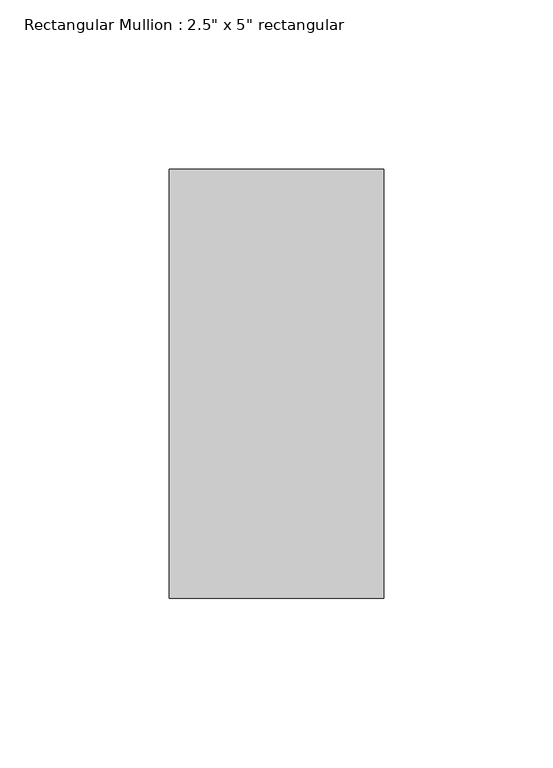
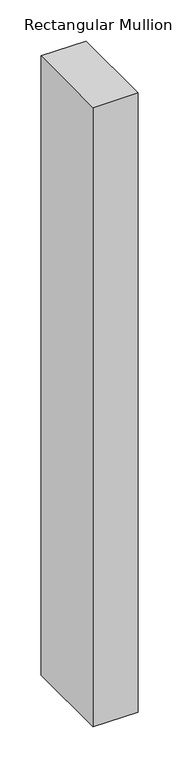
"""IFC4 building model written with IfcOpenShell, lengths in millimetres: member geometry."""

from ifc_helpers import new_model, si_unit, frame, origin, place, context, project, spatial, polyline, outline, extrude, source, transform, mapped, element, save


def member_ff82125d(model_context):
    return source(origin(), model_context, "Body", "SweptSolid", [
        extrude(outline(polyline([(0.0, 63.5), (0.0, -63.5), (-63.5, -63.5), (-63.5, 63.5), (0.0, 63.5)])), frame((0.0, 0.0, -920.75), z_axis=(0.0, 0.0, 1.0), x_axis=(1.0, 0.0, 0.0)), (0.0, 0.0, 1.0), 920.75),
    ])


if __name__ == "__main__":
    model = new_model("IFC4")
    model_context = context("Model", 3, world=origin())
    ifc_project = project(units=[si_unit("LENGTHUNIT", "METRE", prefix="MILLI")], contexts=[model_context])
    site = spatial("IfcSite", under=ifc_project)
    building = spatial("IfcBuilding", under=site)
    placement = place(None, origin())
    member_shape = member_ff82125d(model_context)
    element("IfcMember", 1, ObjectType="Rectangular Mullion : 2.5\" x 5\" rectangular", at=placement, inside=building, context=model_context, shape_type="MappedRepresentation", body=[
        mapped(member_shape, transform((0.0, 0.0, 0.0), x_axis=(1.0, 0.0, 0.0), y_axis=(0.0, 1.0, 0.0), z_axis=(0.0, 0.0, 1.0))),
    ])
    save(model, "model.ifc")

# Revit data of these elements
# Type "Rectangular Mullion : 2.5\" x 5\" rectangular"
#   built-in parameter 1007304 = 0.416667 (stored number, unit not read)
#   built-in parameter 1007301 = 0.104167 (stored number, unit not read)
#   built-in parameter 1007300 = 0.104167 (stored number, unit not read)
# Element 1 (IfcMember, "Rectangular Mullion : 2.5\" x 5\" rectangular")
#   Materials on its faces: "Aluminum"
# Materials
#   "Aluminum": class "Metal", colour RGB 247 247 247, transparency 0, Description = "Aluminum 6061", Cost = 0
